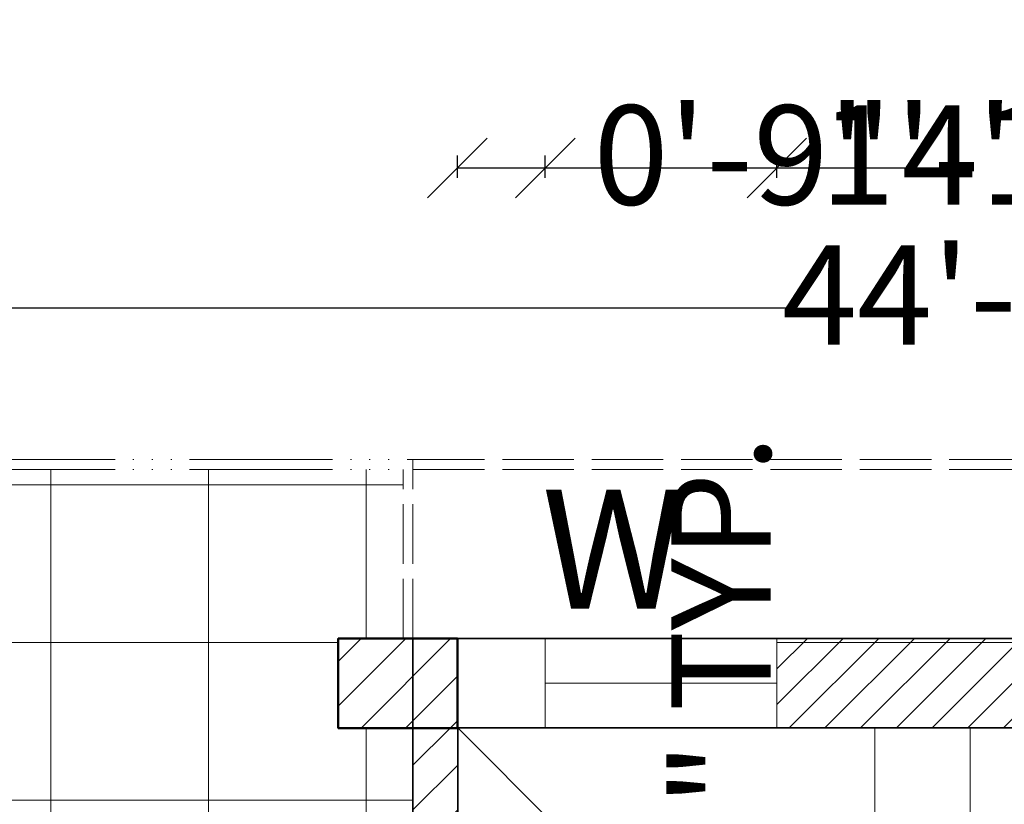
# Model space of a CAD drawing. Units: inches. Extents: x 2036 to 2670, y 319 to 920.
# Tile 10 of 15: x 2251 to 2350, y 841 to 920. Entities that reach past the tile are written whole.
import ezdxf

# ---------------------------------------------------------------- set-up
doc = ezdxf.new("R2010")
doc.units = ezdxf.units.IN
doc.linetypes.add('ACAD_ISO02W100', pattern=[15, 12, -3])
doc.linetypes.add('ACAD_ISO06W100', pattern=[36, 24, -3, 0, -3, 0, -3, 0, -3])
for name, color, linetype, lineweight in [('A-ANNO-DIMS', 2, 'Continuous', 18), ('A-ANNO-TEXT', 7, 'Continuous', 18), ('A-COLS', 7, 'Continuous', 50), ('A-FLOR-EDGE', 5, 'ACAD_ISO06W100', 13), ('A-FLOR-OVHD', 1, 'ACAD_ISO02W100', 13), ('A-FLOR-PATT', 8, 'Continuous', 9), ('A-FLOR-STRS', 7, 'Continuous', 18), ('A-GLAZ', 4, 'Continuous', 18), ('A-WALL', 7, 'Continuous', 35)]:
    doc.layers.add(name, color=color, linetype=linetype, lineweight=lineweight)
doc.layers.add('A-COLS-PATT', color=240, linetype='Continuous', lineweight=13, true_color=0xed1f24)
doc.layers.add('A-WALL-PATT', color=52, linetype='Continuous', lineweight=13, true_color=0xc8c92d)
doc.styles.get("Standard").update_dxf_attribs({"font": 'arial.ttf'})
doc.dimstyles.new('ISO-25', dxfattribs={"dimtxt": 10, "dimasz": 6, "dimexe": 1.25, "dimexo": 0.625, "dimtad": 0, "dimdec": 1, "dimlunit": 3, "dimtxsty": 'Standard', "dimblk": 'OBLIQUE', "dimcen": 2.5, "dimclrd": 94, "dimclre": 94, "dimclrt": 1, "dimadec": 0, "dimazin": 0, "dimtfac": 1, "dimtdec": 1, "dimtmove": 0, "dimatfit": 3, "dimfxl": 1, "dimfxlon": 1, "dimarcsym": 0})

# ---------------------------------------------------------------- blocks, each defined once
blk = doc.blocks.new('_Oblique')
at = {"color": 0, "linetype": 'ByBlock', "lineweight": -2}
blk.add_line((-0.5, -0.5), (0.5, 0.5), dxfattribs=at)
blk = doc.blocks.new('*D10')
at = {"layer": 'A-ANNO-DIMS', "color": 0, "lineweight": -2, "transparency": 16777216}
for p, q in [((2080.735, 889.933), (2080.735, 892.183)), ((2612.735, 889.933), (2612.735, 892.183)), ((2080.735, 890.933), (2328.733, 890.933)), ((2612.735, 890.933), (2364.737, 890.933))]:
    blk.add_line(p, q, dxfattribs=at)
at = {"layer": 'Defpoints', "color": 0, "transparency": 16777216}
for p in [(2612.735, 890.933), (2080.735, 875.685), (2612.735, 875.685)]:
    blk.add_point(p, dxfattribs=at)
at = {"layer": 'A-ANNO-DIMS', "color": 0, "lineweight": -2, "transparency": 16777216, "xscale": 6, "yscale": 6, "zscale": 6, "rotation": 180}
blk.add_blockref('_Oblique', (2080.735, 890.933), dxfattribs=at)
at = {"layer": 'A-ANNO-DIMS', "color": 0, "lineweight": -2, "transparency": 16777216, "xscale": 6, "yscale": 6, "zscale": 6}
blk.add_blockref('_Oblique', (2612.735, 890.933), dxfattribs=at)
at = {"layer": 'A-ANNO-DIMS', "color": 0, "transparency": 16777216, "insert": (2346.735, 890.933), "char_height": 10, "attachment_point": 5}
blk.add_mtext('44\'-4"', dxfattribs=at)
blk = doc.blocks.new('COL-9x12')
blk.add_lwpolyline([(9, 0), (0, 0), (0, 12), (9, 12)], close=True)
blk = doc.blocks.new('*D28')
at = {"layer": 'A-ANNO-DIMS', "color": 94, "lineweight": -2, "transparency": 16777216}
for p, q in [((2323.053, 811.014), (2323.053, 817.014)), ((2322.053, 811.014), (2324.303, 811.014)), ((2323.053, 792.789), (2323.053, 811.014)), ((2322.053, 792.789), (2324.303, 792.789))]:
    blk.add_line(p, q, dxfattribs=at)
at = {"layer": 'Defpoints', "color": 0, "transparency": 16777216}
for p in [(2320.167, 811.014), (2323.053, 811.014), (2320.167, 792.789)]:
    blk.add_point(p, dxfattribs=at)
at = {"layer": 'A-ANNO-DIMS', "color": 94, "lineweight": -2, "transparency": 16777216, "xscale": 6, "yscale": 6, "zscale": 6}
for p, rotation in [((2323.053, 811.014), 90), ((2323.053, 792.789), 270)]:
    blk.add_blockref('_Oblique', p, dxfattribs=dict(at, rotation=rotation))
at = {"layer": 'A-ANNO-DIMS', "color": 1, "transparency": 16777216, "insert": (2323.053, 847.645), "char_height": 10, "attachment_point": 5, "rotation": 90}
blk.add_mtext('1\'-6" TYP.', dxfattribs=at)
blk = doc.blocks.new('*D50')
at = {"layer": 'A-ANNO-DIMS', "color": 94, "lineweight": -2, "transparency": 16777216}
for p, q in [((2295.208, 904.035), (2295.208, 906.285)), ((2304.054, 904.035), (2304.054, 906.285)), ((2295.208, 905.035), (2304.054, 905.035)), ((2304.054, 905.035), (2310.054, 905.035))]:
    blk.add_line(p, q, dxfattribs=at)
at = {"layer": 'Defpoints', "color": 0, "transparency": 16777216}
for p in [(2304.054, 905.035), (2295.208, 857.663), (2304.054, 857.685)]:
    blk.add_point(p, dxfattribs=at)
at = {"layer": 'A-ANNO-DIMS', "color": 94, "lineweight": -2, "transparency": 16777216, "xscale": 6, "yscale": 6, "zscale": 6, "rotation": 180}
blk.add_blockref('_Oblique', (2295.208, 905.035), dxfattribs=at)
at = {"layer": 'A-ANNO-DIMS', "color": 94, "lineweight": -2, "transparency": 16777216, "xscale": 6, "yscale": 6, "zscale": 6}
blk.add_blockref('_Oblique', (2304.054, 905.035), dxfattribs=at)
at = {"layer": 'A-ANNO-DIMS', "color": 1, "transparency": 16777216, "insert": (2323.97, 905.035), "char_height": 10, "attachment_point": 5}
blk.add_mtext('0\'-9"', dxfattribs=at)
blk = doc.blocks.new('*D51')
at = {"layer": 'A-ANNO-DIMS', "color": 94, "lineweight": -2, "transparency": 16777216}
for p, q in [((2304.054, 904.035), (2304.054, 906.285)), ((2327.375, 904.035), (2327.375, 906.285)), ((2304.054, 905.035), (2327.375, 905.035)), ((2327.375, 905.035), (2333.375, 905.035))]:
    blk.add_line(p, q, dxfattribs=at)
at = {"layer": 'Defpoints', "color": 0, "transparency": 16777216}
for p in [(2327.375, 905.035), (2304.054, 857.685), (2327.375, 857.685)]:
    blk.add_point(p, dxfattribs=at)
at = {"layer": 'A-ANNO-DIMS', "color": 94, "lineweight": -2, "transparency": 16777216, "xscale": 6, "yscale": 6, "zscale": 6, "rotation": 180}
blk.add_blockref('_Oblique', (2304.054, 905.035), dxfattribs=at)
at = {"layer": 'A-ANNO-DIMS', "color": 94, "lineweight": -2, "transparency": 16777216, "xscale": 6, "yscale": 6, "zscale": 6}
blk.add_blockref('_Oblique', (2327.375, 905.035), dxfattribs=at)
at = {"layer": 'A-ANNO-DIMS', "color": 1, "transparency": 16777216, "insert": (2362.356, 905.035), "char_height": 10, "attachment_point": 5}
blk.add_mtext('1\'-11 1/2"', dxfattribs=at)
blk = doc.blocks.new('*D52')
at = {"layer": 'A-ANNO-DIMS', "color": 94, "lineweight": -2, "transparency": 16777216}
for p, q in [((2327.375, 904.035), (2327.375, 906.285)), ((2382.618, 904.035), (2382.618, 906.285)), ((2327.375, 905.035), (2340.879, 905.035)), ((2382.618, 905.035), (2369.114, 905.035))]:
    blk.add_line(p, q, dxfattribs=at)
at = {"layer": 'Defpoints', "color": 0, "transparency": 16777216}
for p in [(2382.618, 905.035), (2327.375, 857.685), (2382.618, 857.685)]:
    blk.add_point(p, dxfattribs=at)
at = {"layer": 'A-ANNO-DIMS', "color": 94, "lineweight": -2, "transparency": 16777216, "xscale": 6, "yscale": 6, "zscale": 6, "rotation": 180}
blk.add_blockref('_Oblique', (2327.375, 905.035), dxfattribs=at)
at = {"layer": 'A-ANNO-DIMS', "color": 94, "lineweight": -2, "transparency": 16777216, "xscale": 6, "yscale": 6, "zscale": 6}
blk.add_blockref('_Oblique', (2382.618, 905.035), dxfattribs=at)
at = {"layer": 'A-ANNO-DIMS', "color": 1, "transparency": 16777216, "insert": (2354.996, 905.035), "char_height": 10, "attachment_point": 5}
blk.add_mtext('4\'-7"', dxfattribs=at)

msp = doc.modelspace()

# ---------------------------------------------------------------- hatches: boundary and pattern name
at = {"layer": 'A-COLS-PATT'}
h = msp.add_hatch(dxfattribs=at)
h.set_pattern_fill('ANSI31', color=256)
h.paths.add_polyline_path([(2089.735, 875.685), (2080.735, 875.685), (2080.735, 863.685), (2089.735, 863.685)])
h.paths.add_polyline_path([(2089.735, 821.685), (2080.735, 821.685), (2080.735, 809.685), (2089.735, 809.685)])
h.paths.add_polyline_path([(2089.735, 624.198), (2080.735, 624.198), (2080.735, 612.198), (2089.735, 612.198)])
h.paths.add_polyline_path([(2158.735, 506.685), (2149.735, 506.685), (2149.735, 494.685), (2158.735, 494.685)])
h.paths.add_polyline_path([(2158.735, 617.334), (2149.735, 617.334), (2149.735, 605.334), (2158.735, 605.334)])
h.paths.add_polyline_path([(2158.735, 736.185), (2149.735, 736.185), (2149.735, 724.185), (2158.735, 724.185)])
h.paths.add_polyline_path([(2158.735, 852.814), (2149.735, 852.814), (2149.735, 843.814), (2158.735, 843.814)])
h.paths.add_polyline_path([(2161.735, 852.814), (2158.735, 852.814), (2158.735, 843.814), (2161.735, 843.814)])
h.paths.add_polyline_path([(2295.208, 857.663), (2290.735, 857.663), (2290.735, 848.685), (2295.208, 848.685)])
h.paths.add_polyline_path([(2290.735, 857.663), (2283.208, 857.663), (2283.208, 848.663), (2290.735, 848.663)])
h.paths.add_polyline_path([(2443.623, 857.685), (2431.623, 857.685), (2431.623, 848.685), (2443.623, 848.685)])
h.paths.add_polyline_path([(2561.809, 857.685), (2549.809, 857.685), (2549.809, 848.685), (2561.809, 848.685)])
h.paths.add_polyline_path([(2295.235, 737.646), (2290.735, 737.646), (2290.735, 728.685), (2295.235, 728.685)])
h.paths.add_polyline_path([(2309.268, 612.12), (2297.268, 612.12), (2297.268, 603.12), (2309.268, 603.12)])
h.paths.add_polyline_path([(2282.244, 503.685), (2270.244, 503.685), (2270.244, 494.685), (2282.244, 494.685)])
h.paths.add_polyline_path([(2431.735, 746.091), (2427.235, 746.091), (2427.235, 737.091), (2431.735, 737.091)])
h.paths.add_polyline_path([(2439.235, 746.091), (2431.735, 746.091), (2431.735, 737.091), (2439.235, 737.091)])
h.paths.add_polyline_path([(2596.587, 736.593), (2584.587, 736.593), (2584.587, 727.593), (2596.587, 727.593)])
h.paths.add_polyline_path([(2586.394, 623.705), (2574.394, 623.705), (2574.394, 619.185), (2586.394, 619.185)])
h.paths.add_polyline_path([(2586.394, 619.185), (2574.394, 619.185), (2574.394, 614.705), (2586.394, 614.705)])
h.paths.add_polyline_path([(2438.735, 623.685), (2431.235, 623.685), (2431.235, 619.185), (2438.735, 619.185)])
h.paths.add_polyline_path([(2438.735, 619.185), (2431.235, 619.185), (2431.235, 614.685), (2438.735, 614.685)])
h.paths.add_polyline_path([(2431.235, 623.685), (2426.735, 623.685), (2426.735, 614.685), (2431.235, 614.685), (2431.235, 619.185)])
h.paths.add_polyline_path([(2527.235, 503.685), (2515.235, 503.685), (2515.235, 494.685), (2527.235, 494.685)])
h.paths.add_polyline_path([(2590.311, 503.685), (2578.311, 503.685), (2578.311, 494.685), (2590.311, 494.685)])
at = {"layer": 'A-FLOR-PATT'}
h = msp.add_hatch(dxfattribs=at)
h.set_pattern_fill('ANSI31', color=256, scale=5, angle=135)
h.paths.add_polyline_path([(2290.735, 659.685), (2158.735, 659.685), (2158.735, 582.535), (2158.735, 545.51), (2158.735, 503.685), (2426.735, 503.685), (2426.735, 614.685), (2426.735, 623.685), (2426.735, 628.185), (2431.235, 628.185), (2431.235, 623.685), (2438.735, 623.685), (2438.735, 619.185), (2574.394, 619.185), (2574.394, 623.705), (2586.394, 623.705), (2586.394, 619.185), (2603.735, 619.185), (2603.735, 824.685), (2431.735, 824.685), (2431.735, 746.091), (2439.235, 746.091), (2439.235, 737.091), (2431.735, 737.091), (2431.735, 659.685), (2427.235, 659.685), (2427.235, 739.485), (2383.235, 739.485), (2383.235, 804.685), (2339.235, 804.685), (2339.235, 749.085), (2295.235, 749.085), (2295.235, 737.646), (2295.267, 737.646), (2295.267, 728.646), (2295.213, 728.646, -0.586418), (2272.735, 728.685), (2272.735, 824.685), (2270.113, 824.685), (2270.113, 829.185), (2290.735, 829.185), (2290.735, 848.663), (2283.208, 848.663), (2283.208, 857.663), (2289.735, 857.663), (2289.735, 874.685), (2158.735, 874.685), (2158.735, 852.814), (2161.735, 852.814), (2161.735, 843.814), (2158.735, 843.814), (2158.735, 829.185), (2224.735, 829.185), (2224.735, 800.685), (2182.735, 800.685), (2182.735, 733.415), (2158.735, 733.415), (2158.735, 728.685), (2235.235, 728.685), (2235.235, 714.807), (2230.735, 714.807), (2230.735, 724.185), (2158.735, 724.185), (2158.735, 664.185), (2230.735, 664.185), (2230.735, 678.807), (2235.235, 678.807), (2235.235, 664.185), (2290.735, 664.185)])
h.paths.add_polyline_path([(2309.268, 612.12), (2309.268, 603.12), (2297.268, 603.12), (2297.268, 612.12)], flags=16)
h.paths.add_polyline_path([(2280.116, 639.11), (2280.261, 638.185, -0.414214), (2279.261, 637.185), (2278.761, 637.185), (2279.261, 633.185), (2277.761, 633.185), (2277.261, 637.185), (2269.761, 637.185), (2262.261, 637.185), (2261.761, 633.185), (2260.261, 633.185), (2260.761, 637.185), (2260.261, 637.185, -0.414214), (2259.261, 638.185), (2259.406, 639.11, -0.541164), (2257.761, 641.185), (2260.761, 652.185), (2261.449, 652.185), (2261.527, 652.685), (2262.761, 652.685), (2262.249, 655.244, 0.001913), (2261.761, 655.185), (2259.761, 658.185, -0.15), (2279.761, 658.185), (2277.761, 655.185, 0.001913), (2277.273, 655.244), (2276.761, 652.685), (2277.995, 652.685), (2278.074, 652.185), (2278.761, 652.185), (2281.761, 641.185, -0.541163)], flags=16)
h.paths.add_polyline_path([(2245.984, 639.11), (2246.128, 638.185, -0.414214), (2245.128, 637.185), (2244.628, 637.185), (2245.128, 633.185), (2243.628, 633.185), (2243.128, 637.185), (2235.628, 637.185), (2228.128, 637.185), (2227.628, 633.185), (2226.128, 633.185), (2226.628, 637.185), (2226.128, 637.185, -0.414214), (2225.128, 638.185), (2225.273, 639.11, -0.541164), (2223.628, 641.185), (2226.628, 652.185), (2227.316, 652.185), (2227.394, 652.685), (2228.628, 652.685), (2228.116, 655.244, 0.001913), (2227.628, 655.185), (2225.628, 658.185, -0.15), (2245.628, 658.185), (2243.628, 655.185, 0.001913), (2243.14, 655.244), (2242.628, 652.685), (2243.863, 652.685), (2243.941, 652.185), (2244.628, 652.185), (2247.628, 641.185, -0.541163)], flags=16)
h.paths.add_polyline_path([(2351.59, 515.155, -0.151948), (2279.59, 515.155), (2279.59, 537.685), (2273.59, 537.685), (2273.59, 511.685, 0.190476), (2357.59, 511.685), (2357.59, 537.685), (2351.59, 537.685)])
h.paths.add_polyline_path([(2327.59, 536.127), (2327.59, 517.067), (2303.59, 517.067), (2303.59, 536.127)], flags=16)
h.paths.add_polyline_path([(2213.401, 639.11), (2213.545, 638.185, -0.414214), (2212.545, 637.185), (2212.045, 637.185), (2212.545, 633.185), (2211.045, 633.185), (2210.545, 637.185), (2203.045, 637.185), (2195.545, 637.185), (2195.045, 633.185), (2193.545, 633.185), (2194.045, 637.185), (2193.545, 637.185, -0.414214), (2192.545, 638.185), (2192.69, 639.11, -0.541164), (2191.045, 641.185), (2194.045, 652.185), (2194.733, 652.185), (2194.811, 652.685), (2196.045, 652.685), (2195.534, 655.244, 0.001913), (2195.045, 655.185), (2193.045, 658.185, -0.15), (2213.045, 658.185), (2211.045, 655.185, 0.001913), (2210.557, 655.244), (2210.045, 652.685), (2211.28, 652.685), (2211.358, 652.185), (2212.045, 652.185), (2215.045, 641.185, -0.541163)], flags=16)
h.paths.add_polyline_path([(2368.579, 538.017), (2370.523, 538.017), (2371.17, 532.835), (2380.887, 532.835), (2390.604, 532.835), (2391.252, 538.017), (2393.195, 538.017), (2392.547, 532.835), (2380.887, 532.835), (2368.579, 532.835, 0.414214), (2367.284, 531.54), (2367.471, 530.341, -0.483352), (2369.227, 527.653), (2371.818, 513.401), (2370.118, 513.401), (2370.219, 512.754), (2391.556, 512.754), (2391.657, 513.401), (2389.956, 513.401), (2392.547, 527.653, -1.387427), (2396.434, 527.653), (2392.547, 513.401), (2391.657, 513.401), (2391.556, 512.754), (2389.309, 512.754), (2389.997, 509.367, 0.003796), (2391.252, 509.515), (2393.843, 505.628, -0.15), (2367.931, 505.628), (2370.523, 509.515, 0.003901), (2371.813, 509.363), (2372.466, 512.754), (2370.219, 512.754), (2370.118, 513.401), (2369.227, 513.401), (2365.34, 527.653, -0.541163), (2367.471, 530.341), (2367.284, 531.54, -0.414214), (2368.579, 532.835), (2369.227, 532.835)])
h.paths.add_polyline_path([(2266.738, 538.017), (2266.09, 532.835), (2254.43, 532.835), (2242.122, 532.835, 0.414214), (2240.826, 531.54), (2241.014, 530.341, -0.483352), (2242.77, 527.653), (2245.361, 513.401), (2243.66, 513.401), (2243.762, 512.754), (2265.098, 512.754), (2265.199, 513.401), (2263.499, 513.401), (2266.09, 527.653, -1.387427), (2269.977, 527.653), (2266.09, 513.401), (2265.199, 513.401), (2265.098, 512.754), (2262.851, 512.754), (2263.539, 509.367, 0.003796), (2264.795, 509.515), (2267.386, 505.628, -0.15), (2241.474, 505.628), (2244.065, 509.515, 0.003901), (2245.355, 509.363), (2246.009, 512.754), (2243.762, 512.754), (2243.66, 513.401), (2242.77, 513.401), (2238.883, 527.653, -0.541163), (2241.014, 530.341), (2240.826, 531.54, -0.414214), (2242.122, 532.835), (2242.77, 532.835), (2242.122, 538.017), (2244.065, 538.017), (2244.713, 532.835), (2254.43, 532.835), (2264.147, 532.835), (2264.795, 538.017)])
h.paths.add_polyline_path([(2185.235, 620.355), (2185.235, 618.855), (2181.235, 618.355), (2181.235, 610.855), (2181.235, 603.355), (2185.235, 602.855), (2185.235, 601.355), (2181.235, 601.855), (2181.235, 601.355, -0.414214), (2180.235, 600.355), (2179.31, 600.5, -0.541164), (2177.235, 598.855), (2166.235, 601.855), (2166.235, 602.543), (2165.735, 602.621), (2165.735, 603.855), (2163.176, 603.344, 0.001913), (2163.235, 602.855), (2160.235, 600.855, -0.15), (2160.235, 620.855), (2163.235, 618.855, 0.001913), (2163.176, 618.367), (2165.735, 617.855), (2165.735, 619.09), (2166.235, 619.168), (2166.235, 619.855), (2177.235, 622.855, -0.541163), (2179.31, 621.211), (2180.235, 621.355, -0.414214), (2181.235, 620.355), (2181.235, 619.855)])
h.paths.add_polyline_path([(2470.924, 676.008), (2470.924, 806.129), (2568.515, 806.129), (2568.515, 676.008)], flags=16)
h.paths.add_polyline_path([(2177.738, 677.488), (2161.903, 677.488), (2161.903, 705.848), (2177.738, 705.848)], flags=16)
h.paths.add_polyline_path([(2176.738, 678.488), (2162.903, 678.488), (2162.903, 704.848), (2176.738, 704.848)], flags=0)
h.paths.add_polyline_path([(2175.006, 686.482), (2172.932, 686.482), (2172.932, 690.631), (2170.858, 690.631), (2170.858, 686.482), (2164.634, 686.482), (2164.634, 688.556), (2166.709, 688.556), (2168.783, 688.556), (2168.783, 690.631), (2164.634, 690.631), (2164.634, 696.854), (2166.709, 696.854), (2166.709, 692.705), (2168.783, 692.705), (2168.783, 696.854), (2175.006, 696.854), (2175.006, 694.78), (2170.858, 694.78), (2170.858, 692.705), (2175.006, 692.705)], flags=0)
h.paths.add_polyline_path([(2543.792, 782.707), (2483.937, 782.707), (2483.937, 804.177), (2517.768, 804.177), (2517.768, 782.707), (2521.672, 782.707), (2521.672, 804.177), (2555.503, 804.177), (2555.503, 779.454), (2547.045, 779.454), (2568.515, 757.984), (2543.792, 757.984)], flags=0)
h.paths.add_polyline_path([(2584.587, 727.593), (2584.587, 736.593), (2596.587, 736.593), (2596.587, 727.593)], flags=16)
h.paths.add_polyline_path([(2520.448, 647.035), (2553.788, 647.035), (2553.788, 658.229), (2520.448, 658.229)], flags=24)
h.paths.add_polyline_path([(2299.532, 573.742), (2331.708, 573.742), (2331.708, 584.936), (2299.532, 584.936)], flags=24)
h.paths.add_polyline_path([(2191.593, 685.187), (2212.116, 685.187), (2212.116, 696.382), (2191.593, 696.382)], flags=24)
h.paths.add_polyline_path([(2353.895, 649.863), (2379.08, 649.863), (2379.08, 661.057), (2353.895, 661.057)], flags=24)
h.paths.add_polyline_path([(2214.607, 763.311), (2237.461, 763.311), (2237.461, 779.556), (2214.607, 779.556)], flags=24)
h.paths.add_polyline_path([(2225.093, 819.307), (2269.287, 819.307), (2269.287, 844.035), (2225.093, 844.035)], flags=24)
h.paths.add_polyline_path([(2204.062, 845.043), (2226.916, 845.043), (2226.916, 856.237), (2204.062, 856.237)], flags=24)
h = msp.add_hatch(dxfattribs=at)
h.set_pattern_fill('ANSI31', color=256, scale=5, angle=45)
h.paths.add_polyline_path([(2290.735, 659.685), (2158.735, 659.685), (2158.735, 582.535), (2158.735, 545.51), (2158.735, 503.685), (2426.735, 503.685), (2426.735, 614.685), (2426.735, 623.685), (2426.735, 628.185), (2431.235, 628.185), (2431.235, 623.685), (2438.735, 623.685), (2438.735, 619.185), (2574.394, 619.185), (2574.394, 623.705), (2586.394, 623.705), (2586.394, 619.185), (2603.735, 619.185), (2603.735, 824.685), (2431.735, 824.685), (2431.735, 746.091), (2439.235, 746.091), (2439.235, 737.091), (2431.735, 737.091), (2431.735, 659.685), (2427.235, 659.685), (2427.235, 739.485), (2383.235, 739.485), (2383.235, 804.685), (2339.235, 804.685), (2339.235, 749.085), (2295.235, 749.085), (2295.235, 737.646), (2295.267, 737.646), (2295.267, 728.646), (2295.213, 728.646, -0.586418), (2272.735, 728.685), (2272.735, 824.685), (2270.113, 824.685), (2270.113, 829.185), (2290.735, 829.185), (2290.735, 848.663), (2283.208, 848.663), (2283.208, 857.663), (2289.735, 857.663), (2289.735, 874.685), (2158.735, 874.685), (2158.735, 852.814), (2161.735, 852.814), (2161.735, 843.814), (2158.735, 843.814), (2158.735, 829.185), (2224.735, 829.185), (2224.735, 800.685), (2182.735, 800.685), (2182.735, 733.415), (2158.735, 733.415), (2158.735, 728.685), (2235.235, 728.685), (2235.235, 714.807), (2230.735, 714.807), (2230.735, 724.185), (2158.735, 724.185), (2158.735, 664.185), (2230.735, 664.185), (2230.735, 678.807), (2235.235, 678.807), (2235.235, 664.185), (2290.735, 664.185)])
h.paths.add_polyline_path([(2309.268, 612.12), (2309.268, 603.12), (2297.268, 603.12), (2297.268, 612.12)], flags=16)
h.paths.add_polyline_path([(2280.116, 639.11), (2280.261, 638.185, -0.414214), (2279.261, 637.185), (2278.761, 637.185), (2279.261, 633.185), (2277.761, 633.185), (2277.261, 637.185), (2269.761, 637.185), (2262.261, 637.185), (2261.761, 633.185), (2260.261, 633.185), (2260.761, 637.185), (2260.261, 637.185, -0.414214), (2259.261, 638.185), (2259.406, 639.11, -0.541164), (2257.761, 641.185), (2260.761, 652.185), (2261.449, 652.185), (2261.527, 652.685), (2262.761, 652.685), (2262.249, 655.244, 0.001913), (2261.761, 655.185), (2259.761, 658.185, -0.15), (2279.761, 658.185), (2277.761, 655.185, 0.001913), (2277.273, 655.244), (2276.761, 652.685), (2277.995, 652.685), (2278.074, 652.185), (2278.761, 652.185), (2281.761, 641.185, -0.541163)], flags=16)
h.paths.add_polyline_path([(2245.984, 639.11), (2246.128, 638.185, -0.414214), (2245.128, 637.185), (2244.628, 637.185), (2245.128, 633.185), (2243.628, 633.185), (2243.128, 637.185), (2235.628, 637.185), (2228.128, 637.185), (2227.628, 633.185), (2226.128, 633.185), (2226.628, 637.185), (2226.128, 637.185, -0.414214), (2225.128, 638.185), (2225.273, 639.11, -0.541164), (2223.628, 641.185), (2226.628, 652.185), (2227.316, 652.185), (2227.394, 652.685), (2228.628, 652.685), (2228.116, 655.244, 0.001913), (2227.628, 655.185), (2225.628, 658.185, -0.15), (2245.628, 658.185), (2243.628, 655.185, 0.001913), (2243.14, 655.244), (2242.628, 652.685), (2243.863, 652.685), (2243.941, 652.185), (2244.628, 652.185), (2247.628, 641.185, -0.541163)], flags=16)
h.paths.add_polyline_path([(2351.59, 537.685), (2351.59, 515.155, -0.151948), (2279.59, 515.155), (2279.59, 537.685), (2273.59, 537.685), (2273.59, 511.685, 0.190476), (2357.59, 511.685), (2357.59, 537.685)])
h.paths.add_polyline_path([(2368.579, 538.017), (2370.523, 538.017), (2371.17, 532.835), (2380.887, 532.835), (2390.604, 532.835), (2391.252, 538.017), (2393.195, 538.017), (2392.547, 532.835), (2380.887, 532.835), (2368.579, 532.835, 0.414214), (2367.284, 531.54), (2367.471, 530.341, -0.483352), (2369.227, 527.653), (2371.818, 513.401), (2370.118, 513.401), (2370.219, 512.754), (2391.556, 512.754), (2391.657, 513.401), (2389.956, 513.401), (2392.547, 527.653, -1.387427), (2396.434, 527.653), (2392.547, 513.401), (2391.657, 513.401), (2391.556, 512.754), (2389.309, 512.754), (2389.997, 509.367, 0.003796), (2391.252, 509.515), (2393.843, 505.628, -0.15), (2367.931, 505.628), (2370.523, 509.515, 0.003901), (2371.813, 509.363), (2372.466, 512.754), (2370.219, 512.754), (2370.118, 513.401), (2369.227, 513.401), (2365.34, 527.653, -0.541163), (2367.471, 530.341), (2367.284, 531.54, -0.414214), (2368.579, 532.835), (2369.227, 532.835)])
h.paths.add_polyline_path([(2327.59, 536.127), (2327.59, 517.067), (2303.59, 517.067), (2303.59, 536.127)], flags=16)
h.paths.add_polyline_path([(2470.924, 676.008), (2470.924, 806.129), (2568.515, 806.129), (2568.515, 676.008)], flags=16)
h.paths.add_polyline_path([(2266.738, 538.017), (2266.09, 532.835), (2254.43, 532.835), (2242.122, 532.835, 0.414214), (2240.826, 531.54), (2241.014, 530.341, -0.483352), (2242.77, 527.653), (2245.361, 513.401), (2243.66, 513.401), (2243.762, 512.754), (2265.098, 512.754), (2265.199, 513.401), (2263.499, 513.401), (2266.09, 527.653, -1.387427), (2269.977, 527.653), (2266.09, 513.401), (2265.199, 513.401), (2265.098, 512.754), (2262.851, 512.754), (2263.539, 509.367, 0.003796), (2264.795, 509.515), (2267.386, 505.628, -0.15), (2241.474, 505.628), (2244.065, 509.515, 0.003901), (2245.355, 509.363), (2246.009, 512.754), (2243.762, 512.754), (2243.66, 513.401), (2242.77, 513.401), (2238.883, 527.653, -0.541163), (2241.014, 530.341), (2240.826, 531.54, -0.414214), (2242.122, 532.835), (2242.77, 532.835), (2242.122, 538.017), (2244.065, 538.017), (2244.713, 532.835), (2254.43, 532.835), (2264.147, 532.835), (2264.795, 538.017)])
h.paths.add_polyline_path([(2213.401, 639.11), (2213.545, 638.185, -0.414214), (2212.545, 637.185), (2212.045, 637.185), (2212.545, 633.185), (2211.045, 633.185), (2210.545, 637.185), (2203.045, 637.185), (2195.545, 637.185), (2195.045, 633.185), (2193.545, 633.185), (2194.045, 637.185), (2193.545, 637.185, -0.414214), (2192.545, 638.185), (2192.69, 639.11, -0.541164), (2191.045, 641.185), (2194.045, 652.185), (2194.733, 652.185), (2194.811, 652.685), (2196.045, 652.685), (2195.534, 655.244, 0.001913), (2195.045, 655.185), (2193.045, 658.185, -0.15), (2213.045, 658.185), (2211.045, 655.185, 0.001913), (2210.557, 655.244), (2210.045, 652.685), (2211.28, 652.685), (2211.358, 652.185), (2212.045, 652.185), (2215.045, 641.185, -0.541163)], flags=16)
h.paths.add_polyline_path([(2185.235, 620.355), (2185.235, 618.855), (2181.235, 618.355), (2181.235, 610.855), (2181.235, 603.355), (2185.235, 602.855), (2185.235, 601.355), (2181.235, 601.855), (2181.235, 601.355, -0.414214), (2180.235, 600.355), (2179.31, 600.5, -0.541164), (2177.235, 598.855), (2166.235, 601.855), (2166.235, 602.543), (2165.735, 602.621), (2165.735, 603.855), (2163.176, 603.344, 0.001913), (2163.235, 602.855), (2160.235, 600.855, -0.15), (2160.235, 620.855), (2163.235, 618.855, 0.001913), (2163.176, 618.367), (2165.735, 617.855), (2165.735, 619.09), (2166.235, 619.168), (2166.235, 619.855), (2177.235, 622.855, -0.541163), (2179.31, 621.211), (2180.235, 621.355, -0.414214), (2181.235, 620.355), (2181.235, 619.855)])
h.paths.add_polyline_path([(2177.738, 677.488), (2161.903, 677.488), (2161.903, 705.848), (2177.738, 705.848)], flags=16)
h.paths.add_polyline_path([(2176.738, 678.488), (2162.903, 678.488), (2162.903, 704.848), (2176.738, 704.848)], flags=0)
h.paths.add_polyline_path([(2175.006, 686.482), (2172.932, 686.482), (2172.932, 690.631), (2170.858, 690.631), (2170.858, 686.482), (2164.634, 686.482), (2164.634, 688.556), (2166.709, 688.556), (2168.783, 688.556), (2168.783, 690.631), (2164.634, 690.631), (2164.634, 696.854), (2166.709, 696.854), (2166.709, 692.705), (2168.783, 692.705), (2168.783, 696.854), (2175.006, 696.854), (2175.006, 694.78), (2170.858, 694.78), (2170.858, 692.705), (2175.006, 692.705)], flags=0)
h.paths.add_polyline_path([(2543.792, 782.707), (2483.937, 782.707), (2483.937, 804.177), (2517.768, 804.177), (2517.768, 782.707), (2521.672, 782.707), (2521.672, 804.177), (2555.503, 804.177), (2555.503, 779.454), (2547.045, 779.454), (2568.515, 757.984), (2543.792, 757.984)], flags=0)
h.paths.add_polyline_path([(2584.587, 727.593), (2584.587, 736.593), (2596.587, 736.593), (2596.587, 727.593)], flags=16)
h.paths.add_polyline_path([(2520.448, 647.035), (2553.788, 647.035), (2553.788, 658.229), (2520.448, 658.229)], flags=24)
h.paths.add_polyline_path([(2299.532, 573.742), (2331.708, 573.742), (2331.708, 584.936), (2299.532, 584.936)], flags=24)
h.paths.add_polyline_path([(2191.593, 685.187), (2212.116, 685.187), (2212.116, 696.382), (2191.593, 696.382)], flags=24)
h.paths.add_polyline_path([(2353.895, 649.863), (2379.08, 649.863), (2379.08, 661.057), (2353.895, 661.057)], flags=24)
h.paths.add_polyline_path([(2214.607, 763.311), (2237.461, 763.311), (2237.461, 779.556), (2214.607, 779.556)], flags=24)
h.paths.add_polyline_path([(2225.093, 819.307), (2269.287, 819.307), (2269.287, 844.035), (2225.093, 844.035)], flags=24)
h.paths.add_polyline_path([(2204.062, 845.043), (2226.916, 845.043), (2226.916, 856.237), (2204.062, 856.237)], flags=24)
at = {"layer": 'A-WALL-PATT'}
h = msp.add_hatch(dxfattribs=at)
h.set_pattern_fill('ANSI31', color=256)
h.paths.add_polyline_path([(2089.735, 863.685), (2080.735, 863.685), (2080.735, 821.685), (2089.735, 821.685)])
h.paths.add_polyline_path([(2089.735, 809.685), (2080.735, 809.685), (2080.735, 624.198), (2089.735, 624.198), (2089.735, 707.685), (2089.735, 767.685)])
h.paths.add_polyline_path([(2149.735, 818.685), (2089.735, 818.685), (2089.735, 809.685), (2149.735, 809.685)])
h.paths.add_polyline_path([(2158.735, 875.685), (2089.735, 875.685), (2089.735, 866.685), (2149.735, 866.685), (2149.735, 852.814), (2158.735, 852.814)])
h.paths.add_polyline_path([(2158.735, 843.814), (2149.735, 843.814), (2149.735, 736.185), (2158.735, 736.185), (2158.735, 824.685)])
h.paths.add_polyline_path([(2181.313, 829.185), (2158.735, 829.185), (2158.735, 824.685), (2181.313, 824.685)])
h.paths.add_polyline_path([(2224.735, 829.185), (2212.718, 829.185), (2212.718, 824.685), (2224.735, 824.685)])
h.paths.add_polyline_path([(2177.022, 503.685), (2158.735, 503.685), (2158.735, 494.685), (2177.022, 494.685)])
h.paths.add_polyline_path([(2158.735, 664.185), (2158.735, 680.019), (2149.735, 680.019), (2149.735, 617.334), (2158.735, 617.334)])
h.paths.add_polyline_path([(2158.735, 724.185), (2149.735, 724.185), (2149.735, 704.019), (2158.735, 704.019)])
h.paths.add_polyline_path([(2235.235, 728.685), (2158.735, 728.685), (2158.735, 724.185), (2230.735, 724.185), (2230.735, 714.807), (2235.235, 714.807)])
h.paths.add_polyline_path([(2290.735, 664.185), (2235.235, 664.185), (2235.235, 678.807), (2230.735, 678.807), (2230.735, 664.185), (2158.735, 664.185), (2158.735, 659.685), (2290.735, 659.685)])
h.paths.add_polyline_path([(2270.244, 503.685), (2227.168, 503.685), (2227.168, 494.685), (2270.244, 494.685)])
h.paths.add_polyline_path([(2515.235, 503.685), (2380.887, 503.685), (2380.887, 494.685), (2515.235, 494.685)])
h.paths.add_polyline_path([(2292.211, 503.685), (2282.244, 503.685), (2282.244, 494.685), (2292.211, 494.685)])
h.paths.add_polyline_path([(2578.311, 503.685), (2527.235, 503.685), (2527.235, 494.685), (2578.311, 494.685)])
h.paths.add_polyline_path([(2603.735, 503.685), (2590.311, 503.685), (2590.311, 494.685), (2603.735, 494.685)])
h.paths.add_polyline_path([(2612.735, 503.685), (2603.735, 503.685), (2603.735, 494.685), (2612.735, 494.685)])
h.paths.add_polyline_path([(2549.809, 857.685), (2443.623, 857.685), (2443.623, 848.685), (2549.809, 848.685)])
h.paths.add_polyline_path([(2295.235, 848.663), (2290.735, 848.663), (2290.735, 829.185), (2270.113, 829.185), (2270.113, 824.685), (2290.735, 824.685), (2290.735, 737.646), (2295.235, 737.646)])
h.paths.add_polyline_path([(2431.735, 737.091), (2427.235, 737.091), (2427.235, 659.685), (2431.735, 659.685)])
h.paths.add_polyline_path([(2431.735, 848.685), (2427.235, 848.685), (2427.235, 746.091), (2431.735, 746.091)])
h.paths.add_polyline_path([(2574.394, 619.185), (2495.46, 619.185), (2495.46, 614.685), (2574.394, 614.685)])
h.paths.add_polyline_path([(2461.836, 619.185), (2438.735, 619.185), (2438.735, 614.685), (2461.836, 614.685)])
h.paths.add_polyline_path([(2603.735, 619.185), (2586.394, 619.185), (2586.394, 614.685), (2603.735, 614.685)], flags=17)
h = msp.add_hatch(dxfattribs=at)
h.set_pattern_fill('ANSI31', color=256, scale=3, angle=135)
h.paths.add_polyline_path([(2382.618, 857.685), (2327.375, 857.685), (2327.375, 848.685), (2382.618, 848.685)])
h.paths.add_polyline_path([(2431.623, 857.685), (2414.791, 857.685), (2414.791, 848.685), (2427.235, 848.685), (2431.623, 848.685)])
h = msp.add_hatch(dxfattribs=at)
h.set_pattern_fill('ANSI31', color=256, scale=0.8)
h.paths.add_polyline_path([(2431.623, 857.685), (2414.791, 857.685), (2414.791, 848.685), (2427.235, 848.685), (2431.623, 848.685)])
h.paths.add_polyline_path([(2382.618, 857.685), (2327.375, 857.685), (2327.375, 848.685), (2382.618, 848.685)])

# ---------------------------------------------------------------- linework, layer by layer
at = {"layer": 'A-FLOR-EDGE', "ltscale": 0.6}
for p, q in [((2158.735, 875.685), (2290.735, 875.685)), ((2158.735, 874.685), (2289.735, 874.685))]:
    msp.add_line(p, q, dxfattribs=at)
at = {"layer": 'A-FLOR-OVHD', "ltscale": 0.6}
for p, q in [((2290.735, 875.685), (2612.735, 875.685)), ((2290.735, 874.685), (2612.735, 874.685))]:
    msp.add_line(p, q, dxfattribs=at)
at = {"layer": 'A-FLOR-OVHD', "ltscale": 0.5}
for p, q in [((2290.735, 857.685), (2290.735, 875.685)), ((2289.735, 857.685), (2289.735, 874.685))]:
    msp.add_line(p, q, dxfattribs=at)
at = {"layer": 'A-FLOR-STRS'}
for p, q in [((2337.235, 806.685), (2295.235, 848.685)), ((2337.235, 806.685), (2337.235, 848.685)), ((2346.835, 806.685), (2346.835, 848.685))]:
    msp.add_line(p, q, dxfattribs=at)
at = {"layer": 'A-GLAZ'}
for p, q in [((2304.054, 857.685), (2304.054, 848.685)), ((2327.375, 857.685), (2327.375, 848.685)), ((2304.054, 853.185), (2327.375, 853.185))]:
    msp.add_line(p, q, dxfattribs=at)
at = {"layer": 'A-WALL'}
for p, q in [((2612.735, 857.685), (2290.735, 857.685)), ((2290.735, 829.185), (2290.735, 857.685)), ((2295.235, 848.685), (2290.735, 848.685)), ((2295.235, 728.685), (2295.235, 848.685)), ((2427.235, 848.685), (2295.235, 848.685))]:
    msp.add_line(p, q, dxfattribs=at)

# ---------------------------------------------------------------- block references
at = {"layer": 'A-COLS', "rotation": 89.999999999998}
msp.add_blockref('COL-9x12', (2295.208, 848.663), dxfattribs=at)

# ---------------------------------------------------------------- texts
at = {"layer": 'A-ANNO-TEXT', "insert": (2303.693, 872.665), "char_height": 12, "attachment_point": 1}
msp.add_mtext_dynamic_manual_height_columns('W', width=27.69719, gutter_width=12.5, heights=[0], dxfattribs=at)

# ---------------------------------------------------------------- dimensions: what is measured, and where the dimension line sits
at = {"layer": 'A-ANNO-DIMS'}
for base, p1, p2, override, picture, middle in [((2327.375, 905.035), (2304.054, 857.685), (2327.375, 857.685), {"dimdec": 1, "dimlfac": 1, "dimrnd": 0, "dimzin": 1, "dimdsep": 46, "dimlunit": 4, "dimfrac": 2}, '*D51', (2362.356, 905.035)), ((2304.054, 905.035), (2295.208, 857.663), (2304.054, 857.685), {"dimdec": 1, "dimlfac": 1, "dimrnd": 0, "dimzin": 1, "dimdsep": 46, "dimlunit": 4, "dimfrac": 2}, '*D50', (2323.97, 905.035)), ((2382.618, 905.035), (2327.375, 857.685), (2382.618, 857.685), {"dimdec": 1, "dimlfac": 1, "dimrnd": 0, "dimzin": 1, "dimdsep": 46, "dimlunit": 4, "dimfrac": 2}, '*D52', (2354.996, 905.035)), ((2612.735, 890.933), (2080.735, 875.685), (2612.735, 875.685), {"dimclrd": 0, "dimclre": 0, "dimclrt": 0}, '*D10', (2346.735, 890.933))]:
    dim = msp.add_linear_dim(base=base, p1=p1, p2=p2, dimstyle='ISO-25', override=override, dxfattribs=at)
    dim.commit()
    dim.dimension.update_dxf_attribs({"geometry": picture, "text_midpoint": middle})
dim = msp.add_linear_dim(base=(2323.053, 811.014), p1=(2320.167, 792.789), p2=(2320.167, 811.014), angle=90, text='<> TYP.', dimstyle='ISO-25', override={"dimdec": 1, "dimlfac": 1, "dimrnd": 0, "dimzin": 1, "dimdsep": 46, "dimlunit": 4, "dimfrac": 2}, dxfattribs=at)
dim.commit()
dim.dimension.update_dxf_attribs({"geometry": '*D28', "text_midpoint": (2323.053, 847.645)})

doc.saveas('drawing.dxf')
